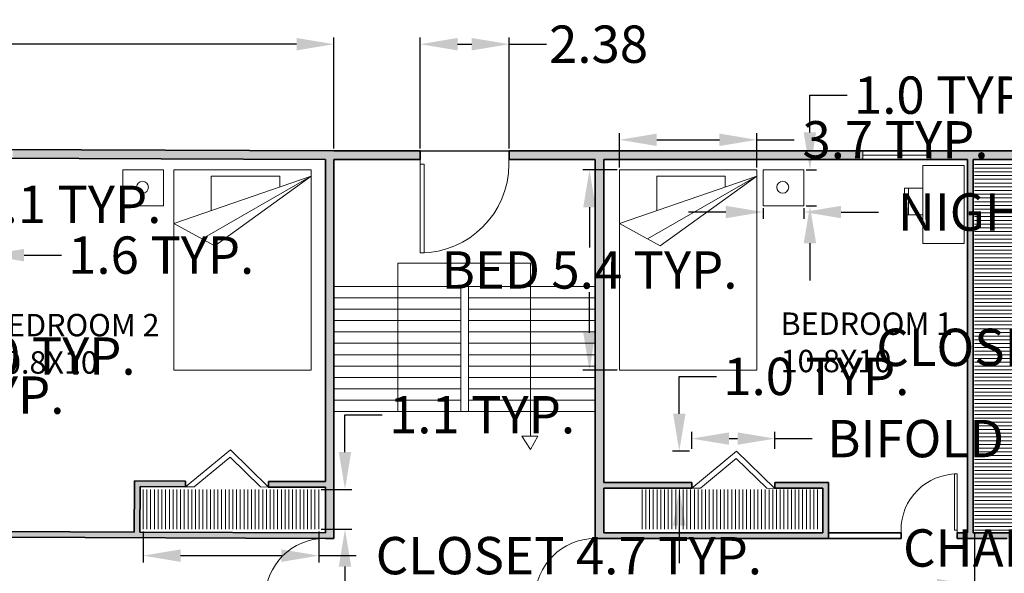
# Model space of a CAD drawing. Units: metres. Extents: x 25.1 to 96.1, y 24.3 to 71.3.
# Tile 4 of 5: x 45.8 to 72.2, y 56.5 to 71.3. Entities that reach past the tile are written whole.
import ezdxf

# ---------------------------------------------------------------- set-up
doc = ezdxf.new("R2010")
doc.units = ezdxf.units.M
doc.header["$MEASUREMENT"] = 0
for name, color, linetype, lineweight in [('A-ANNO-SYMB', 7, 'Continuous', 13), ('A-AREA-IDEN', 1, 'Continuous', 18), ('A-FLOR-CASE', 8, 'Continuous', 18), ('A-FLOR-STRS', 7, 'Continuous', 18), ('A-GLAZ', 4, 'Continuous', 18), ('A-WALL', 7, 'Continuous', 35), ('A-WALL-PATT', 252, 'Continuous', 13), ('dimension', 80, 'Continuous', 18), ('door', 17, 'Continuous', 18), ('furniture', 163, 'Continuous', 18)]:
    doc.layers.add(name, color=color, linetype=linetype, lineweight=lineweight)
doc.styles.get("Standard").update_dxf_attribs({"font": 'arial.ttf'})
doc.dimstyles.get("Standard").update_dxf_attribs({"dimtxt": 1, "dimasz": 1, "dimexe": 0.18, "dimexo": 0.0625, "dimgap": 0.09, "dimtad": 0, "dimtih": 1, "dimtoh": 1, "dimdec": 1, "dimzin": 0, "dimdsep": 46, "dimtxsty": 'Standard', "dimcen": 0.09, "dimadec": 0, "dimazin": 0, "dimtfac": 1, "dimtdec": 1, "dimtofl": 0, "dimtmove": 0, "dimatfit": 3, "dimfxl": 1, "dimtolj": 1, "dimtzin": 0, "dimarcsym": 0})

# ---------------------------------------------------------------- blocks, each defined once
blk = doc.blocks.new('bb')
for p, q in [((37.478, 19.517), (33.802, 18.246)), ((37.478, 19.517), (34.553, 17.835)), ((34.896, 17.647), (37.478, 19.517)), ((33.802, 18.246), (34.896, 17.647))]:
    blk.add_line(p, q)
blk.add_lwpolyline([(37.478, 19.683), (33.802, 19.683), (33.802, 14.322), (37.478, 14.322)], close=True)
blk.add_lwpolyline([(34.801, 18.591), (34.801, 19.517), (36.636, 19.517), (36.636, 19.226)])
blk = doc.blocks.new('tt')
for points in [[(27.188, 19.803), (28.295, 19.803), (28.295, 17.712), (27.188, 17.712)], [(28.295, 19.193), (28.681, 19.193), (28.681, 18.478), (28.295, 18.478)], [(28.681, 19.193), (28.789, 19.193), (28.789, 18.478), (28.681, 18.478)]]:
    blk.add_lwpolyline(points, close=True)
blk = doc.blocks.new('dd')
for p, q in [((35.313, 12.188), (34.11, 11.198)), ((36.337, 11.189), (35.313, 12.188)), ((35.304, 11.986), (34.345, 11.197)), ((36.121, 11.19), (35.304, 11.986)), ((34.11, 11.198), (34.345, 11.197)), ((36.121, 11.19), (36.337, 11.189))]:
    blk.add_line(p, q)
blk = doc.blocks.new('f')
at = {"layer": 'furniture'}
for p, q in [((25.769, 19.917), (26.843, 19.917)), ((25.769, 19.817), (26.843, 19.817)), ((25.769, 19.717), (26.843, 19.717)), ((25.769, 19.617), (26.843, 19.617)), ((25.769, 19.517), (26.843, 19.517)), ((25.769, 19.417), (26.843, 19.417)), ((25.769, 19.317), (26.843, 19.317)), ((25.769, 19.217), (26.843, 19.217)), ((25.769, 19.117), (26.843, 19.117)), ((25.769, 19.017), (26.843, 19.017)), ((25.769, 18.917), (26.843, 18.917)), ((25.769, 18.817), (26.843, 18.817)), ((25.769, 18.717), (26.843, 18.717)), ((25.769, 18.617), (26.843, 18.617)), ((25.769, 18.517), (26.843, 18.517)), ((25.769, 18.417), (26.843, 18.417)), ((25.769, 18.317), (26.843, 18.317)), ((25.769, 18.217), (26.843, 18.217)), ((25.769, 18.117), (26.843, 18.117)), ((25.769, 18.017), (26.843, 18.017)), ((25.769, 17.917), (26.843, 17.917)), ((25.769, 17.817), (26.843, 17.817)), ((25.769, 17.717), (26.843, 17.717)), ((25.769, 17.617), (26.843, 17.617)), ((25.769, 17.517), (26.843, 17.517)), ((25.769, 17.417), (26.843, 17.417)), ((25.769, 17.317), (26.843, 17.317)), ((25.769, 17.217), (26.843, 17.217)), ((25.769, 17.117), (26.843, 17.117)), ((25.769, 17.017), (26.843, 17.017)), ((25.769, 16.917), (26.843, 16.917)), ((25.769, 16.817), (26.843, 16.817)), ((25.769, 16.717), (26.843, 16.717)), ((25.769, 16.617), (26.843, 16.617)), ((25.769, 16.517), (26.843, 16.517)), ((25.769, 16.417), (26.843, 16.417)), ((25.769, 16.317), (26.843, 16.317)), ((25.769, 16.217), (26.843, 16.217)), ((25.769, 16.117), (26.843, 16.117)), ((25.769, 16.017), (26.843, 16.017)), ((25.769, 15.917), (26.843, 15.917)), ((25.769, 15.817), (26.843, 15.817)), ((25.769, 15.717), (26.843, 15.717)), ((25.769, 15.617), (26.843, 15.617)), ((25.769, 15.517), (26.843, 15.517)), ((25.769, 15.417), (26.843, 15.417)), ((25.769, 15.317), (26.843, 15.317)), ((25.769, 15.217), (26.843, 15.217)), ((25.769, 15.117), (26.843, 15.117)), ((25.769, 15.017), (26.843, 15.017)), ((25.769, 14.917), (26.843, 14.917)), ((25.769, 14.817), (26.843, 14.817)), ((25.769, 14.717), (26.843, 14.717)), ((25.769, 14.617), (26.843, 14.617)), ((25.769, 14.517), (26.843, 14.517)), ((25.769, 14.417), (26.843, 14.417)), ((25.769, 14.317), (26.843, 14.317)), ((25.769, 14.217), (26.843, 14.217)), ((25.769, 14.117), (26.843, 14.117)), ((25.769, 14.017), (26.843, 14.017)), ((25.769, 13.917), (26.843, 13.917)), ((25.769, 13.817), (26.843, 13.817)), ((25.769, 13.717), (26.843, 13.717)), ((25.769, 13.617), (26.843, 13.617)), ((25.769, 13.517), (26.843, 13.517)), ((25.769, 13.417), (26.843, 13.417)), ((25.769, 13.317), (26.843, 13.317)), ((25.769, 13.217), (26.843, 13.217)), ((25.769, 13.117), (26.843, 13.117)), ((25.769, 13.017), (26.843, 13.017)), ((25.769, 12.917), (26.843, 12.917)), ((25.769, 12.817), (26.843, 12.817)), ((25.769, 12.717), (26.843, 12.717)), ((25.769, 12.617), (26.843, 12.617)), ((25.769, 12.517), (26.843, 12.517)), ((25.769, 12.417), (26.843, 12.417)), ((25.769, 12.317), (26.843, 12.317)), ((25.769, 12.217), (26.843, 12.217)), ((25.769, 12.117), (26.843, 12.117)), ((25.769, 12.017), (26.843, 12.017)), ((25.769, 11.917), (26.843, 11.917)), ((25.769, 11.817), (26.843, 11.817)), ((25.769, 11.717), (26.843, 11.717)), ((25.769, 11.617), (26.843, 11.617)), ((25.769, 11.517), (26.843, 11.517)), ((25.769, 11.417), (26.843, 11.417)), ((25.769, 11.317), (26.843, 11.317)), ((25.769, 11.217), (26.843, 11.217)), ((25.769, 11.117), (26.843, 11.117)), ((25.769, 11.017), (26.843, 11.017)), ((25.769, 10.917), (26.843, 10.917)), ((25.769, 10.817), (26.843, 10.817)), ((25.769, 10.717), (26.843, 10.717)), ((25.769, 10.617), (26.843, 10.617)), ((25.769, 10.517), (26.843, 10.517)), ((25.769, 10.417), (26.843, 10.417)), ((25.769, 10.317), (26.843, 10.317)), ((25.769, 10.217), (26.843, 10.217)), ((25.769, 10.117), (26.843, 10.117))]:
    blk.add_line(p, q, dxfattribs=at)
blk = doc.blocks.new('ff')
at = {"layer": 'furniture'}
for p, q in [((32.978, 11.126), (32.978, 10.056)), ((33.078, 11.126), (33.078, 10.056)), ((33.178, 11.126), (33.178, 10.056)), ((33.278, 11.126), (33.278, 10.056)), ((33.378, 11.126), (33.378, 10.056)), ((33.478, 11.126), (33.478, 10.056)), ((33.578, 11.126), (33.578, 10.056)), ((33.678, 11.126), (33.678, 10.056)), ((33.778, 11.126), (33.778, 10.056)), ((33.878, 11.126), (33.878, 10.056)), ((33.978, 11.126), (33.978, 10.056)), ((34.078, 11.126), (34.078, 10.056)), ((34.178, 11.126), (34.178, 10.056)), ((34.278, 11.126), (34.278, 10.056)), ((34.378, 11.126), (34.378, 10.056)), ((34.478, 11.126), (34.478, 10.056)), ((34.578, 11.126), (34.578, 10.056)), ((34.678, 11.126), (34.678, 10.056)), ((34.778, 11.126), (34.778, 10.056)), ((34.878, 11.126), (34.878, 10.056)), ((34.978, 11.126), (34.978, 10.056)), ((35.078, 11.126), (35.078, 10.056)), ((35.178, 11.126), (35.178, 10.056)), ((35.278, 11.126), (35.278, 10.056)), ((35.378, 11.126), (35.378, 10.056)), ((35.478, 11.126), (35.478, 10.056)), ((35.578, 11.126), (35.578, 10.056)), ((35.678, 11.126), (35.678, 10.056)), ((35.778, 11.126), (35.778, 10.056)), ((35.878, 11.126), (35.878, 10.056)), ((35.978, 11.126), (35.978, 10.056)), ((36.078, 11.126), (36.078, 10.056)), ((36.178, 11.126), (36.178, 10.056)), ((36.278, 11.126), (36.278, 10.056)), ((36.378, 11.126), (36.378, 10.056)), ((36.478, 11.126), (36.478, 10.056)), ((36.578, 11.126), (36.578, 10.056)), ((36.678, 11.126), (36.678, 10.056)), ((36.778, 11.126), (36.778, 10.056)), ((36.878, 11.126), (36.878, 10.056)), ((36.978, 11.126), (36.978, 10.056)), ((37.078, 11.126), (37.078, 10.056)), ((37.178, 11.126), (37.178, 10.056)), ((37.278, 11.126), (37.278, 10.056)), ((37.378, 11.126), (37.378, 10.056)), ((37.478, 11.126), (37.478, 10.056)), ((37.578, 11.126), (37.578, 10.056)), ((37.678, 11.126), (37.678, 10.056))]:
    blk.add_line(p, q, dxfattribs=at)
blk = doc.blocks.new('*U22')
for p, q in [((0, 0), (0, -6)), ((40, 0), (40, -6))]:
    blk.add_line(p, q)
blk.add_lwpolyline([(0, 0), (0, 40), (1.75, 40), (1.75, 0)], close=True)
blk.add_arc((0, 0), 40, 0, 90)
blk = doc.blocks.new('BEDROOM-NIGHTSTAND')
blk.add_lwpolyline([(1.09, 0.966), (0, 0.966), (0, 0), (1.09, 0)], close=True)
blk.add_circle((0.525, 0.501), 0.159)
blk = doc.blocks.new('STAIR-PAIRED-FLIGHTS')
for p, q in [((0, 3.353), (7, 3.353)), ((3.4, 3.353), (3.4, 0)), ((3.6, 3.353), (3.6, 0)), ((0, 3.048), (3.4, 3.048)), ((3.6, 3.048), (7, 3.048)), ((0, 2.743), (3.4, 2.743)), ((3.6, 2.743), (7, 2.743)), ((0, 2.438), (3.4, 2.438)), ((3.6, 2.438), (7, 2.438)), ((0, 2.133), (3.4, 2.133)), ((3.6, 2.133), (7, 2.133)), ((0, 1.829), (3.4, 1.829)), ((3.6, 1.829), (7, 1.829)), ((0, 1.524), (3.4, 1.524)), ((3.6, 1.524), (7, 1.524)), ((0, 1.219), (3.4, 1.219)), ((3.6, 1.219), (7, 1.219)), ((0, 0.914), (3.4, 0.914)), ((3.6, 0.914), (7, 0.914)), ((0, 0.609), (3.4, 0.609)), ((3.6, 0.609), (7, 0.609)), ((0, 0.305), (3.4, 0.305)), ((3.6, 0.305), (7, 0.305)), ((0, 0), (7, 0))]:
    blk.add_line(p, q)
blk = doc.blocks.new('*D32')
at = {"layer": 'Defpoints', "color": 0, "transparency": 16777216}
for p in [(41.726, 62.046), (41.726, 60.436), (41.967, 60.436)]:
    blk.add_point(p, dxfattribs=at)
at = {"layer": 'dimension', "color": 0, "lineweight": -2, "transparency": 16777216}
for p, q in [((41.967, 63.046), (41.967, 64.046)), ((41.788, 62.046), (42.147, 62.046)), ((41.788, 60.436), (42.147, 60.436)), ((41.967, 59.436), (41.967, 58.436))]:
    blk.add_line(p, q, dxfattribs=at)
at = {"layer": 'dimension', "color": 0, "transparency": 16777216}
for points in [[(41.801, 63.046), (42.134, 63.046), (41.967, 62.046)], [(41.801, 59.436), (42.134, 59.436), (41.967, 60.436)]]:
    blk.add_solid(points, dxfattribs=at)
at = {"layer": 'dimension', "color": 0, "transparency": 16777216, "insert": (41.967, 61.241), "char_height": 1, "attachment_point": 5}
blk.add_mtext('\\A1;BIFOLD 1.6 TYP.', dxfattribs=at)
blk = doc.blocks.new('*D33')
at = {"layer": 'Defpoints', "color": 0, "transparency": 16777216}
for p in [(41.726, 62.287), (40.771, 62.046), (41.726, 62.046)]:
    blk.add_point(p, dxfattribs=at)
at = {"layer": 'dimension', "color": 0, "lineweight": -2, "transparency": 16777216}
for p, q in [((39.771, 62.287), (38.771, 62.287)), ((40.771, 62.108), (40.771, 62.467)), ((41.726, 62.108), (41.726, 62.467)), ((42.726, 62.287), (43.726, 62.287))]:
    blk.add_line(p, q, dxfattribs=at)
at = {"layer": 'dimension', "color": 0, "transparency": 16777216}
for points in [[(39.771, 62.454), (39.771, 62.121), (40.771, 62.287)], [(42.726, 62.454), (42.726, 62.121), (41.726, 62.287)]]:
    blk.add_solid(points, dxfattribs=at)
at = {"layer": 'dimension', "color": 0, "transparency": 16777216, "insert": (46.397, 62.287), "char_height": 1, "attachment_point": 5}
blk.add_mtext('\\A1;1.0 TYP.', dxfattribs=at)
blk = doc.blocks.new('*D36')
at = {"layer": 'Defpoints', "color": 0, "transparency": 16777216}
for p in [(72.431, 67.419), (73.901, 67.419), (72.431, 57.619)]:
    blk.add_point(p, dxfattribs=at)
at = {"layer": 'dimension', "color": 0, "lineweight": -2, "transparency": 16777216}
for p, q in [((72.494, 67.419), (74.081, 67.419)), ((73.901, 66.419), (73.901, 63.126)), ((73.901, 58.619), (73.901, 61.912)), ((72.494, 57.619), (74.081, 57.619))]:
    blk.add_line(p, q, dxfattribs=at)
at = {"layer": 'dimension', "color": 0, "transparency": 16777216}
for points in [[(73.735, 66.419), (74.068, 66.419), (73.901, 67.419)], [(73.735, 58.619), (74.068, 58.619), (73.901, 57.619)]]:
    blk.add_solid(points, dxfattribs=at)
at = {"layer": 'dimension', "color": 0, "transparency": 16777216, "insert": (73.901, 62.519), "char_height": 1, "attachment_point": 5}
blk.add_mtext('\\A1;CLOSET 9.8 TYP.', dxfattribs=at)
blk = doc.blocks.new('*D37')
at = {"layer": 'Defpoints', "color": 0, "transparency": 16777216}
for p in [(71.357, 57.619), (72.431, 57.619), (72.431, 56.149)]:
    blk.add_point(p, dxfattribs=at)
at = {"layer": 'dimension', "color": 0, "lineweight": -2, "transparency": 16777216}
for p, q in [((71.357, 57.557), (71.357, 55.969)), ((72.431, 57.557), (72.431, 55.969)), ((70.357, 56.149), (69.357, 56.149)), ((73.431, 56.149), (74.431, 56.149))]:
    blk.add_line(p, q, dxfattribs=at)
at = {"layer": 'dimension', "color": 0, "transparency": 16777216}
for points in [[(70.357, 56.316), (70.357, 55.982), (71.357, 56.149)], [(73.431, 56.316), (73.431, 55.982), (72.431, 56.149)]]:
    blk.add_solid(points, dxfattribs=at)
at = {"layer": 'dimension', "color": 0, "transparency": 16777216, "insert": (77.102, 56.149), "char_height": 1, "attachment_point": 5}
blk.add_mtext('\\A1;1.1 TYP.', dxfattribs=at)
blk = doc.blocks.new('*D48')
at = {"layer": 'Defpoints', "color": 0, "transparency": 16777216}
for p in [(80.148, 57.146), (80.148, 56.81), (82.383, 56.81)]:
    blk.add_point(p, dxfattribs=at)
at = {"layer": 'dimension', "color": 0, "lineweight": -2, "transparency": 16777216}
for p, q in [((80.148, 56.873), (80.148, 57.326)), ((82.383, 56.873), (82.383, 57.326)), ((80.148, 57.146), (79.148, 57.146)), ((81.383, 57.146), (81.148, 57.146))]:
    blk.add_line(p, q, dxfattribs=at)
at = {"layer": 'dimension', "color": 0, "transparency": 16777216}
for points in [[(81.148, 57.312), (81.148, 56.979), (80.148, 57.146)], [(81.383, 57.312), (81.383, 56.979), (82.383, 57.146)]]:
    blk.add_solid(points, dxfattribs=at)
at = {"layer": 'dimension', "color": 0, "transparency": 16777216, "insert": (74.068, 57.146), "char_height": 1, "attachment_point": 5}
blk.add_mtext('\\A1;CHAIR 2.2 TYP.', dxfattribs=at)
blk = doc.blocks.new('*D50')
at = {"layer": 'Defpoints', "color": 0, "transparency": 16777216}
for p in [(61.045, 67.273), (61.849, 67.273), (61.849, 61.911)]:
    blk.add_point(p, dxfattribs=at)
at = {"layer": 'dimension', "color": 0, "lineweight": -2, "transparency": 16777216}
for p, q in [((61.787, 67.273), (60.865, 67.273)), ((61.045, 66.273), (61.045, 65.191)), ((61.045, 62.911), (61.045, 63.994)), ((61.787, 61.911), (60.865, 61.911))]:
    blk.add_line(p, q, dxfattribs=at)
at = {"layer": 'dimension', "color": 0, "transparency": 16777216}
for points in [[(60.878, 66.273), (61.211, 66.273), (61.045, 67.273)], [(60.878, 62.911), (61.211, 62.911), (61.045, 61.911)]]:
    blk.add_solid(points, dxfattribs=at)
at = {"layer": 'dimension', "color": 0, "transparency": 16777216, "insert": (61.045, 64.592), "char_height": 1, "attachment_point": 5}
blk.add_mtext('\\A1;BED 5.4 TYP.', dxfattribs=at)
blk = doc.blocks.new('*D51')
at = {"layer": 'Defpoints', "color": 0, "transparency": 16777216}
for p in [(65.524, 68.077), (61.849, 67.273), (65.524, 67.273)]:
    blk.add_point(p, dxfattribs=at)
at = {"layer": 'dimension', "color": 0, "lineweight": -2, "transparency": 16777216}
for p, q in [((61.849, 67.335), (61.849, 68.257)), ((62.849, 68.077), (64.524, 68.077)), ((65.524, 67.335), (65.524, 68.257)), ((65.524, 68.077), (66.524, 68.077))]:
    blk.add_line(p, q, dxfattribs=at)
at = {"layer": 'dimension', "color": 0, "transparency": 16777216}
for points in [[(62.849, 68.244), (62.849, 67.91), (61.849, 68.077)], [(64.524, 68.244), (64.524, 67.91), (65.524, 68.077)]]:
    blk.add_solid(points, dxfattribs=at)
at = {"layer": 'dimension', "color": 0, "transparency": 16777216, "insert": (69.242, 68.077), "char_height": 1, "attachment_point": 5}
blk.add_mtext('\\A1;3.7 TYP.', dxfattribs=at)
blk = doc.blocks.new('*D52')
at = {"layer": 'Defpoints', "color": 0, "transparency": 16777216}
for p in [(44.903, 67.393), (45.216, 67.393), (44.903, 65.302)]:
    blk.add_point(p, dxfattribs=at)
at = {"layer": 'dimension', "color": 0, "lineweight": -2, "transparency": 16777216}
for p, q in [((45.216, 68.393), (45.216, 69.393)), ((44.965, 67.393), (45.396, 67.393)), ((44.965, 65.302), (45.396, 65.302)), ((45.216, 64.302), (45.216, 63.302))]:
    blk.add_line(p, q, dxfattribs=at)
at = {"layer": 'dimension', "color": 0, "transparency": 16777216}
for points in [[(45.05, 68.393), (45.383, 68.393), (45.216, 67.393)], [(45.05, 64.302), (45.383, 64.302), (45.216, 65.302)]]:
    blk.add_solid(points, dxfattribs=at)
at = {"layer": 'dimension', "color": 0, "transparency": 16777216, "insert": (45.216, 66.348), "char_height": 1, "attachment_point": 5}
blk.add_mtext('\\A1;DESK 2.1 TYP.', dxfattribs=at)
blk = doc.blocks.new('*D53')
at = {"layer": 'Defpoints', "color": 0, "transparency": 16777216}
for p in [(43.302, 65.302), (44.903, 65.302), (44.903, 64.989)]:
    blk.add_point(p, dxfattribs=at)
at = {"layer": 'dimension', "color": 0, "lineweight": -2, "transparency": 16777216}
for p, q in [((43.302, 65.24), (43.302, 64.809)), ((44.903, 65.24), (44.903, 64.809)), ((42.302, 64.989), (41.302, 64.989)), ((45.903, 64.989), (46.903, 64.989))]:
    blk.add_line(p, q, dxfattribs=at)
at = {"layer": 'dimension', "color": 0, "transparency": 16777216}
for points in [[(42.302, 65.155), (42.302, 64.822), (43.302, 64.989)], [(45.903, 65.155), (45.903, 64.822), (44.903, 64.989)]]:
    blk.add_solid(points, dxfattribs=at)
at = {"layer": 'dimension', "color": 0, "transparency": 16777216, "insert": (49.574, 64.989), "char_height": 1, "attachment_point": 5}
blk.add_mtext('\\A1;1.6 TYP.', dxfattribs=at)
blk = doc.blocks.new('*D54')
at = {"layer": 'Defpoints', "color": 0, "transparency": 16777216}
for p in [(66.011, 60.075), (63.784, 59.741), (66.011, 59.741)]:
    blk.add_point(p, dxfattribs=at)
at = {"layer": 'dimension', "color": 0, "lineweight": -2, "transparency": 16777216}
for p, q in [((63.784, 59.804), (63.784, 60.255)), ((66.011, 59.804), (66.011, 60.255)), ((64.784, 60.075), (65.011, 60.075)), ((66.011, 60.075), (67.011, 60.075))]:
    blk.add_line(p, q, dxfattribs=at)
at = {"layer": 'dimension', "color": 0, "transparency": 16777216}
for points in [[(64.784, 60.242), (64.784, 59.909), (63.784, 60.075)], [(65.011, 60.242), (65.011, 59.909), (66.011, 60.075)]]:
    blk.add_solid(points, dxfattribs=at)
at = {"layer": 'dimension', "color": 0, "transparency": 16777216, "insert": (72.424, 60.075), "char_height": 1, "attachment_point": 5}
blk.add_mtext('\\A1;BIFOLD 2.2 TYP.', dxfattribs=at)
blk = doc.blocks.new('*D55')
at = {"layer": 'Defpoints', "color": 0, "transparency": 16777216}
for p in [(63.45, 59.741), (63.784, 59.741), (63.784, 58.742)]:
    blk.add_point(p, dxfattribs=at)
at = {"layer": 'dimension', "color": 0, "lineweight": -2, "transparency": 16777216}
for p, q in [((63.45, 60.741), (63.45, 61.741)), ((63.45, 61.741), (64.45, 61.741)), ((63.722, 59.741), (63.27, 59.741)), ((63.722, 58.742), (63.27, 58.742)), ((63.45, 57.742), (63.45, 56.742))]:
    blk.add_line(p, q, dxfattribs=at)
at = {"layer": 'dimension', "color": 0, "transparency": 16777216}
for points in [[(63.284, 60.741), (63.617, 60.741), (63.45, 59.741)], [(63.284, 57.742), (63.617, 57.742), (63.45, 58.742)]]:
    blk.add_solid(points, dxfattribs=at)
at = {"layer": 'dimension', "color": 0, "transparency": 16777216, "insert": (67.121, 61.741), "char_height": 1, "attachment_point": 5}
blk.add_mtext('\\A1;1.0 TYP.', dxfattribs=at)
blk = doc.blocks.new('*D56')
at = {"layer": 'Defpoints', "color": 0, "transparency": 16777216}
for p in [(49.092, 57.646), (53.792, 57.646), (53.792, 56.941)]:
    blk.add_point(p, dxfattribs=at)
at = {"layer": 'dimension', "color": 0, "lineweight": -2, "transparency": 16777216}
for p, q in [((49.092, 57.584), (49.092, 56.761)), ((53.792, 57.584), (53.792, 56.761)), ((50.092, 56.941), (52.792, 56.941)), ((53.792, 56.941), (54.792, 56.941))]:
    blk.add_line(p, q, dxfattribs=at)
at = {"layer": 'dimension', "color": 0, "transparency": 16777216}
for points in [[(50.092, 57.108), (50.092, 56.774), (49.092, 56.941)], [(52.792, 57.108), (52.792, 56.774), (53.792, 56.941)]]:
    blk.add_solid(points, dxfattribs=at)
at = {"layer": 'dimension', "color": 0, "transparency": 16777216, "insert": (60.493, 56.941), "char_height": 1, "attachment_point": 5}
blk.add_mtext('\\A1;CLOSET 4.7 TYP.', dxfattribs=at)
blk = doc.blocks.new('*D57')
at = {"layer": 'Defpoints', "color": 0, "transparency": 16777216}
for p in [(53.792, 58.716), (54.497, 58.716), (53.792, 57.646)]:
    blk.add_point(p, dxfattribs=at)
at = {"layer": 'dimension', "color": 0, "lineweight": -2, "transparency": 16777216}
for p, q in [((54.497, 59.716), (54.497, 60.716)), ((54.497, 60.716), (55.497, 60.716)), ((53.855, 58.716), (54.677, 58.716)), ((53.855, 57.646), (54.677, 57.646)), ((54.497, 56.646), (54.497, 55.646))]:
    blk.add_line(p, q, dxfattribs=at)
at = {"layer": 'dimension', "color": 0, "transparency": 16777216}
for points in [[(54.331, 59.716), (54.664, 59.716), (54.497, 58.716)], [(54.331, 56.646), (54.664, 56.646), (54.497, 57.646)]]:
    blk.add_solid(points, dxfattribs=at)
at = {"layer": 'dimension', "color": 0, "transparency": 16777216, "insert": (58.168, 60.716), "char_height": 1, "attachment_point": 5}
blk.add_mtext('\\A1;1.1 TYP.', dxfattribs=at)
blk = doc.blocks.new('*D70')
at = {"layer": 'Defpoints', "color": 0, "transparency": 16777216}
for p in [(65.697, 66.307), (66.786, 66.307), (66.786, 66.143)]:
    blk.add_point(p, dxfattribs=at)
at = {"layer": 'dimension', "color": 0, "lineweight": -2, "transparency": 16777216}
for p, q in [((65.697, 66.244), (65.697, 65.963)), ((66.786, 66.244), (66.786, 65.963)), ((64.697, 66.143), (63.697, 66.143)), ((67.786, 66.143), (68.786, 66.143))]:
    blk.add_line(p, q, dxfattribs=at)
at = {"layer": 'dimension', "color": 0, "transparency": 16777216}
for points in [[(64.697, 66.31), (64.697, 65.977), (65.697, 66.143)], [(67.786, 66.31), (67.786, 65.977), (66.786, 66.143)]]:
    blk.add_solid(points, dxfattribs=at)
at = {"layer": 'dimension', "color": 0, "transparency": 16777216, "insert": (76.214, 66.143), "char_height": 1, "attachment_point": 5}
blk.add_mtext('\\A1;NIGHTSTAND 1.1 TYP.', dxfattribs=at)
blk = doc.blocks.new('*D71')
at = {"layer": 'Defpoints', "color": 0, "transparency": 16777216}
for p in [(66.786, 67.273), (66.95, 67.273), (66.786, 66.307)]:
    blk.add_point(p, dxfattribs=at)
at = {"layer": 'dimension', "color": 0, "lineweight": -2, "transparency": 16777216}
for p, q in [((66.95, 68.273), (66.95, 69.273)), ((66.95, 69.273), (67.95, 69.273)), ((66.849, 67.273), (67.13, 67.273)), ((66.849, 66.307), (67.13, 66.307)), ((66.95, 65.307), (66.95, 64.307))]:
    blk.add_line(p, q, dxfattribs=at)
at = {"layer": 'dimension', "color": 0, "transparency": 16777216}
for points in [[(66.783, 68.273), (67.116, 68.273), (66.95, 67.273)], [(66.783, 65.307), (67.116, 65.307), (66.95, 66.307)]]:
    blk.add_solid(points, dxfattribs=at)
at = {"layer": 'dimension', "color": 0, "transparency": 16777216, "insert": (70.621, 69.273), "char_height": 1, "attachment_point": 5}
blk.add_mtext('\\A1;1.0 TYP.', dxfattribs=at)
blk = doc.blocks.new('*D81')
at = {"layer": 'Defpoints', "color": 0, "transparency": 16777216}
for p in [(54.201, 70.638), (32.047, 67.873), (54.201, 67.782)]:
    blk.add_point(p, dxfattribs=at)
at = {"layer": 'dimension', "color": 0, "lineweight": -2, "transparency": 16777216}
for p, q in [((32.047, 67.935), (32.047, 70.818)), ((54.201, 67.844), (54.201, 70.818)), ((33.047, 70.638), (40.952, 70.638)), ((53.201, 70.638), (45.296, 70.638))]:
    blk.add_line(p, q, dxfattribs=at)
at = {"layer": 'dimension', "color": 0, "transparency": 16777216}
for points in [[(33.047, 70.804), (33.047, 70.471), (32.047, 70.638)], [(53.201, 70.804), (53.201, 70.471), (54.201, 70.638)]]:
    blk.add_solid(points, dxfattribs=at)
at = {"layer": 'dimension', "color": 0, "transparency": 16777216, "insert": (43.124, 70.638), "char_height": 1, "attachment_point": 5}
blk.add_mtext('\\A1;22.154', dxfattribs=at)
blk = doc.blocks.new('*D85')
at = {"layer": 'Defpoints', "color": 0, "transparency": 16777216}
for p in [(54.201, 67.782), (86.176, 67.782), (54.201, 54.198)]:
    blk.add_point(p, dxfattribs=at)
at = {"layer": 'dimension', "color": 0, "lineweight": -2, "transparency": 16777216}
for p, q in [((54.263, 67.782), (86.356, 67.782)), ((86.176, 66.782), (86.176, 61.59)), ((86.176, 55.198), (86.176, 60.389)), ((54.263, 54.198), (86.356, 54.198))]:
    blk.add_line(p, q, dxfattribs=at)
at = {"layer": 'dimension', "color": 0, "transparency": 16777216}
for points in [[(86.009, 66.782), (86.342, 66.782), (86.176, 67.782)], [(86.009, 55.198), (86.342, 55.198), (86.176, 54.198)]]:
    blk.add_solid(points, dxfattribs=at)
at = {"layer": 'dimension', "color": 0, "transparency": 16777216, "insert": (86.176, 60.99), "char_height": 1, "attachment_point": 5}
blk.add_mtext('\\A1;13.584', dxfattribs=at)
blk = doc.blocks.new('*D86')
at = {"layer": 'Defpoints', "color": 0, "transparency": 16777216}
for p in [(58.891, 70.638), (56.511, 67.782), (58.891, 67.782)]:
    blk.add_point(p, dxfattribs=at)
at = {"layer": 'dimension', "color": 0, "lineweight": -2, "transparency": 16777216}
for p, q in [((56.511, 67.844), (56.511, 70.818)), ((58.891, 67.844), (58.891, 70.818)), ((57.511, 70.638), (57.891, 70.638)), ((58.891, 70.638), (59.891, 70.638))]:
    blk.add_line(p, q, dxfattribs=at)
at = {"layer": 'dimension', "color": 0, "transparency": 16777216}
for points in [[(57.511, 70.804), (57.511, 70.471), (56.511, 70.638)], [(57.891, 70.804), (57.891, 70.471), (58.891, 70.638)]]:
    blk.add_solid(points, dxfattribs=at)
at = {"layer": 'dimension', "color": 0, "transparency": 16777216, "insert": (61.289, 70.638), "char_height": 1, "attachment_point": 5}
blk.add_mtext('\\A1;2.38', dxfattribs=at)

msp = doc.modelspace()

# ---------------------------------------------------------------- hatches: boundary and pattern name
at = {"layer": 'A-WALL-PATT'}
h = msp.add_hatch(color=256, dxfattribs=at)
h.dxf.hatch_style = 1
h.paths.add_polyline_path([(32.2705, 66.2918), (32.0405, 66.2928), (31.9902, 54.0475), (31.9902, 50.7969), (32.2202, 50.7969), (32.2202, 54.0475), (42.8202, 54.0475), (42.8202, 52.5275), (42.9702, 52.5275), (42.9702, 54.0475), (43.1708, 54.0475), (43.1708, 54.1975), (32.2208, 54.1975)])
h.paths.add_polyline_path([(32.8404, 67.8694), (32.047, 67.8727), (32.0456, 67.5128), (32.2756, 67.5118), (32.2761, 67.6417), (32.8395, 67.6394)])
h.paths.add_polyline_path([(43.7857, 67.8244), (34.0604, 67.8644), (34.0595, 67.6344), (41.6508, 67.6032), (41.6508, 63.9251), (41.8008, 63.9251), (41.8008, 67.6026), (43.0208, 67.5975), (43.0208, 57.5975), (41.8008, 57.6025), (41.8008, 60.436), (41.6508, 60.436), (41.6508, 57.4531), (43.8592, 57.444), (43.8592, 57.594), (43.1708, 57.5968), (43.1708, 67.5969), (43.7848, 67.5944)])
h.paths.add_polyline_path([(56.5108, 67.7816), (54.2008, 67.7816), (45.5957, 67.8169), (45.5947, 67.5869), (53.9708, 67.5525), (53.9708, 58.9224), (52.4515, 58.9287), (52.4508, 58.779), (52.4512, 58.7787), (53.9708, 58.7724), (53.9708, 57.5524), (49.0027, 57.5728), (49.0077, 58.7928), (50.2244, 58.7878), (50.2244, 58.9378), (48.8584, 58.9435), (48.8577, 58.7935), (48.8527, 57.5735), (45.4006, 57.5877), (45.4006, 57.4377), (53.9634, 57.4024), (54.2008, 57.4024), (54.2008, 67.5516), (56.5108, 67.5516)])
h.paths.add_polyline_path([(68.3657, 67.7816), (58.8908, 67.7816), (58.8908, 67.5516), (61.2008, 67.5516), (61.2008, 57.4016), (61.4308, 57.4016), (67.4455, 57.4016), (67.4455, 58.9016), (66.0112, 58.9016), (66.0112, 58.7516), (67.2955, 58.7516), (67.2955, 57.5516), (61.4308, 57.5516), (61.4308, 58.7516), (63.7844, 58.7516), (63.7844, 58.9016), (61.4308, 58.9016), (61.4308, 67.5516), (68.3657, 67.5516)])
h = msp.add_hatch(color=256, dxfattribs=at)
h.dxf.hatch_style = 1
h.paths.add_polyline_path([(72.6908, 67.5516), (81.5153, 67.5516), (81.5153, 67.7816), (70.1857, 67.7816), (70.1857, 67.5516), (71.1708, 67.5516), (71.1708, 57.5516), (70.8915, 57.5516), (70.8915, 57.4016), (72.2308, 57.4016), (72.6908, 57.4016), (72.6908, 60.436), (72.6185, 60.436), (72.5408, 60.436), (72.5408, 57.5516), (71.3208, 57.5516), (71.3208, 67.5516), (72.5408, 67.5516), (72.5408, 63.9324), (72.6908, 63.9324)])
h.paths.add_polyline_path([(83.4108, 67.7816), (82.7353, 67.7816), (82.7353, 67.5516), (83.1808, 67.5516), (83.1808, 67.3623), (83.4108, 67.3623)])

# ---------------------------------------------------------------- linework, layer by layer
at = {"layer": 'A-ANNO-SYMB'}
for p, q in [((55.9141, 60.7988), (55.9141, 64.7745)), ((55.9141, 64.7745), (59.4668, 64.7745)), ((59.4668, 64.7745), (59.4668, 60.1419)), ((59.4668, 60.1419), (59.2341, 60.1419)), ((59.2341, 60.1419), (59.4668, 59.7862)), ((59.6622, 60.1419), (59.4255, 60.1419)), ((59.4668, 59.7862), (59.6622, 60.1419))]:
    msp.add_line(p, q, dxfattribs=at)
at = {"layer": 'A-GLAZ'}
for p, q in [((68.3657, 67.5516), (68.3657, 67.7816)), ((70.1857, 67.5516), (70.1857, 67.7816)), ((68.3657, 67.6666), (70.1857, 67.6666))]:
    msp.add_line(p, q, dxfattribs=at)
at = {"layer": 'A-WALL'}
for p, q in [((32.047, 67.8727), (54.2008, 67.7816)), ((54.2008, 67.7816), (56.5108, 67.7816)), ((56.5108, 67.5516), (56.5108, 67.7816)), ((58.8908, 67.7816), (83.4108, 67.7816)), ((58.8908, 67.5516), (58.8908, 67.7816)), ((43.1708, 67.5969), (53.9708, 67.5525)), ((53.9708, 67.5525), (53.9708, 58.9224)), ((54.2008, 67.5516), (54.2008, 57.4024)), ((54.2008, 67.5516), (56.5108, 67.5516)), ((58.8908, 67.5516), (61.2008, 67.5516)), ((61.2008, 67.5516), (61.2008, 57.4016)), ((61.4308, 67.5516), (61.4308, 58.9016)), ((61.4308, 67.5516), (71.1708, 67.5516)), ((71.1708, 67.5516), (71.1708, 57.5516)), ((71.3208, 67.5516), (71.3208, 57.5516)), ((71.3208, 67.5516), (72.5408, 67.5516)), ((48.8577, 58.7935), (48.8584, 58.9435)), ((48.8584, 58.9435), (50.2244, 58.9378)), ((50.2244, 58.7878), (50.2244, 58.9378)), ((52.4515, 58.9287), (52.4508, 58.7787)), ((52.4515, 58.9287), (53.9764, 58.9224)), ((61.4308, 58.9016), (63.7844, 58.9016)), ((63.7844, 58.7516), (63.7844, 58.9016)), ((66.0112, 58.7424), (66.0112, 58.9016)), ((66.0112, 58.9016), (67.4455, 58.9016)), ((67.4455, 57.4016), (67.4455, 58.9016)), ((48.8527, 57.5735), (48.8577, 58.7935)), ((49.0027, 57.5728), (49.0077, 58.7928)), ((49.0077, 58.7928), (50.2244, 58.7878)), ((52.4508, 58.7787), (53.9758, 58.7724)), ((53.9708, 58.7724), (53.9708, 57.5524)), ((61.4308, 58.7516), (63.7844, 58.7516)), ((61.4308, 58.7516), (61.4308, 57.5516)), ((66.0112, 58.7516), (67.2955, 58.7516)), ((67.2955, 57.5516), (67.2955, 58.7516)), ((45.3998, 57.5877), (48.8527, 57.5735)), ((49.0027, 57.5728), (53.9708, 57.5524)), ((61.4308, 57.5516), (67.2955, 57.5516)), ((67.4455, 57.5516), (69.3915, 57.5516)), ((69.3915, 57.5516), (69.3915, 57.4016)), ((69.3915, 57.5516), (69.3915, 57.4016)), ((70.8915, 57.5516), (70.8915, 57.4016)), ((70.8915, 57.5516), (71.1708, 57.5516)), ((71.3208, 57.5516), (72.5408, 57.5516)), ((45.3992, 57.4377), (53.9708, 57.4024)), ((53.9708, 57.4024), (54.2008, 57.4024)), ((61.4308, 57.4016), (61.2008, 57.4016)), ((61.4308, 57.4016), (69.3915, 57.4016)), ((70.8915, 57.4016), (72.2308, 57.4016))]:
    msp.add_line(p, q, dxfattribs=at)
for points in [[(54.2008, 57.4024), (53.9708, 57.4024)], [(61.2008, 57.4024), (61.2008, 57.399)], [(61.4308, 57.399), (61.4308, 57.4024)]]:
    msp.add_lwpolyline(points, dxfattribs=at)

# ---------------------------------------------------------------- block references
at = {"layer": 'A-FLOR-CASE'}
for name, p in [('f', (45.5881, 47.5021)), ('ff', (16.1141, 47.5898)), ('ff', (29.4771, 47.5898))]:
    msp.add_blockref(name, p, dxfattribs=at)
at = {"layer": 'A-FLOR-STRS'}
msp.add_blockref('STAIR-PAIRED-FLIGHTS', (54.201, 60.799), dxfattribs=at)
at = {"layer": 'door'}
for p, xscale, yscale, zscale, rotation in [((56.5108, 67.4253), -0.059373656253378, 0.059373656253378, 0.059373656253378, 180), ((70.8915, 57.6268), -0.0375410848744283, 0.0375410848744283, 0.0375410848744283, 359.9999999999992), ((53.9604, 55.8), 0.0400617254265443, 0.0400617254265443, 0.0400617254265443, 90), ((61.1909, 55.8), 0.0399749143269108, 0.0399749143269108, 0.0399749143269108, 90)]:
    msp.add_blockref('*U22', p, dxfattribs=dict(at, xscale=xscale, yscale=yscale, zscale=zscale, rotation=rotation))
for p in [(16.1141, 47.5898), (29.6742, 47.5535)]:
    msp.add_blockref('dd', p, dxfattribs=at)
at = {"layer": 'furniture'}
for name, p in [('BEDROOM-NIGHTSTAND', (48.548, 66.307)), ('bb', (16.1141, 47.5898)), ('bb', (28.0467, 47.5898)), ('BEDROOM-NIGHTSTAND', (65.6967, 66.307))]:
    msp.add_blockref(name, p, dxfattribs=at)
at = {"layer": 'furniture', "xscale": -1}
msp.add_blockref('tt', (98.2722, 47.5898), dxfattribs=at)

# ---------------------------------------------------------------- texts
at = {"layer": 'A-AREA-IDEN', "char_height": 0.6, "attachment_point": 1}
for s, insert in [('BEDROOM 2\\P10.8X10', (44.9092, 63.415)), ('BEDROOM 1\\P10.8X10', (66.1635, 63.453))]:
    msp.add_mtext_dynamic_manual_height_columns(s, width=5.007262, gutter_width=1, heights=[0], dxfattribs=dict(at, insert=insert))

# ---------------------------------------------------------------- dimensions: what is measured, and where the dimension line sits
at = {"layer": 'dimension'}
for base, p1, p2, override, picture, middle in [((54.2008, 70.6377), (32.047, 67.8727), (54.2008, 67.7816), {"dimdec": 3, "dimlfac": 1, "dimrnd": 0, "dimzin": 0, "dimdsep": 46, "dimlunit": 2}, '*D81', (43.1239, 70.6377)), ((58.8908, 70.6377), (56.5108, 67.7816), (58.8908, 67.7816), {"dimdec": 2, "dimlfac": 1, "dimrnd": 0, "dimzin": 0, "dimdsep": 46, "dimlunit": 2}, '*D86', (61.2891, 70.6377))]:
    dim = msp.add_linear_dim(base=base, p1=p1, p2=p2, dimstyle='Standard', override=override, dxfattribs=at)
    dim.commit()
    dim.dimension.update_dxf_attribs({"geometry": picture, "text_midpoint": middle})
for base, p1, p2, angle, text, picture, middle in [((66.9497, 67.2729), (66.7863, 66.3066), (66.7863, 67.2729), 90, '<> TYP.', '*D71', (70.6206, 69.2729)), ((45.2164, 67.393), (44.9028, 65.3022), (44.9028, 67.393), 90, 'DESK <> TYP.', '*D52', (45.2164, 66.3476)), ((61.0448, 67.2729), (61.8491, 61.9114), (61.8491, 67.2729), 90, 'BED <> TYP.', '*D50', (61.0448, 64.5922)), ((73.9012, 67.4191), (72.4312, 57.6191), (72.4312, 67.4191), 90, 'CLOSET <> TYP.', '*D36', (73.9012, 62.5191)), ((41.9673, 60.436), (41.7258, 62.0459), (41.7258, 60.436), 270, 'BIFOLD <> TYP.', '*D32', (41.9673, 61.241)), ((63.4504, 59.7412), (63.7844, 58.7424), (63.7844, 59.7412), 90, '<> TYP.', '*D55', (67.1213, 61.7412)), ((54.4975, 58.7156), (53.7925, 57.6461), (53.7925, 58.7156), 90, '<> TYP.', '*D57', (58.1683, 60.7156)), ((80.1479, 57.1455), (82.383, 56.8102), (80.1479, 56.8102), 180, 'CHAIR <> TYP.', '*D48', (74.0685, 57.1455))]:
    dim = msp.add_linear_dim(base=base, p1=p1, p2=p2, angle=angle, text=text, dimstyle='Standard', override={"dimdec": 1, "dimlfac": 1, "dimrnd": 0, "dimzin": 0, "dimdsep": 46, "dimlunit": 2}, dxfattribs=at)
    dim.commit()
    dim.dimension.update_dxf_attribs({"geometry": picture, "text_midpoint": middle})
for base, p1, p2, text, picture, middle in [((65.5244, 68.0771), (61.8491, 67.2729), (65.5244, 67.2729), '<> TYP.', '*D51', (69.2419, 68.0771)), ((66.7863, 66.1432), (65.6965, 66.3066), (66.7863, 66.3066), 'NIGHTSTAND <> TYP.', '*D70', (76.2143, 66.1432)), ((44.9028, 64.9886), (43.3025, 65.3022), (44.9028, 65.3022), '<> TYP.', '*D53', (49.5736, 64.9886)), ((41.7258, 62.2874), (40.7713, 62.0459), (41.7258, 62.0459), '<> TYP.', '*D33', (46.3966, 62.2874)), ((66.0112, 60.0752), (63.7844, 59.7412), (66.0112, 59.7412), 'BIFOLD <> TYP.', '*D54', (72.4239, 60.0752)), ((53.7925, 56.9411), (49.0925, 57.6461), (53.7925, 57.6461), 'CLOSET <> TYP.', '*D56', (60.4933, 56.9411)), ((72.4312, 56.1491), (71.3574, 57.6191), (72.4312, 57.6191), '<> TYP.', '*D37', (77.1021, 56.1491))]:
    dim = msp.add_linear_dim(base=base, p1=p1, p2=p2, text=text, dimstyle='Standard', override={"dimdec": 1, "dimlfac": 1, "dimrnd": 0, "dimzin": 0, "dimdsep": 46, "dimlunit": 2}, dxfattribs=at)
    dim.commit()
    dim.dimension.update_dxf_attribs({"geometry": picture, "text_midpoint": middle})
dim = msp.add_linear_dim(base=(86.1758, 67.7816), p1=(54.2008, 54.1975), p2=(54.2008, 67.7816), angle=90, dimstyle='Standard', override={"dimdec": 3, "dimlfac": 1, "dimrnd": 0, "dimzin": 0, "dimdsep": 46, "dimlunit": 2}, dxfattribs=at)
dim.commit()
dim.dimension.update_dxf_attribs({"geometry": '*D85', "text_midpoint": (86.1758, 60.9895)})

doc.saveas('drawing.dxf')
